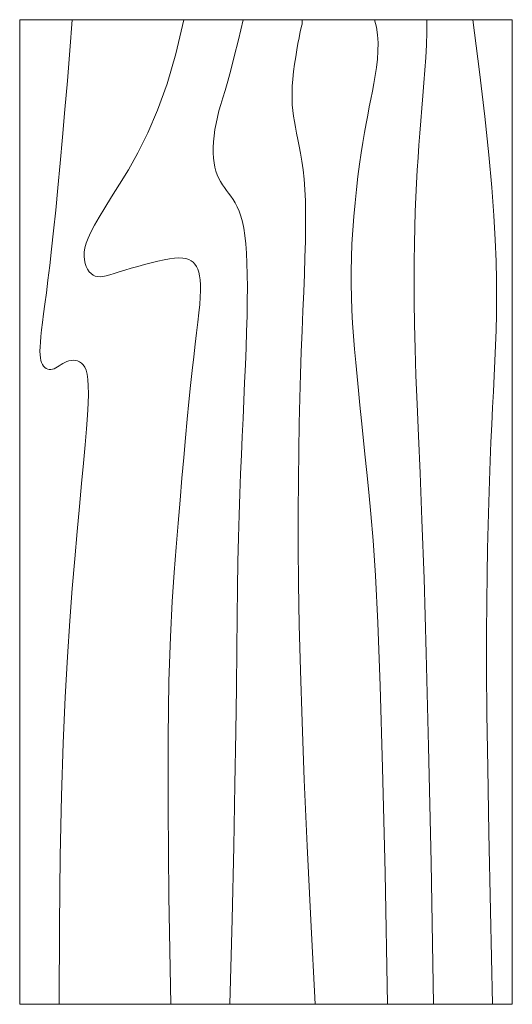
# Model space of a CAD drawing. Units: inches. Extents: x 3209 to 7144, y 1281 to 3076.
# Tile 5 of 5: x 7114 to 7144, y 3016 to 3076. Entities that reach past the tile are written whole.
import ezdxf

# ---------------------------------------------------------------- set-up
doc = ezdxf.new("R2010")
doc.units = ezdxf.units.IN
doc.layers.add('A-FURN', color=8, linetype='Continuous', lineweight=18)

# ---------------------------------------------------------------- blocks, each defined once
blk = doc.blocks.new('Table - Rectangular Woodgrain 60 x 30 in.')
for p, q in [((0, 0), (0, -30)), ((60, 0), (0, 0)), ((60, -30), (60, 0)), ((0, -30), (60, -30))]:
    blk.add_line(p, q)
for points in [[(0, -2.4), (4.8155, -2.418), (9.0302, -2.4688), (12.709, -2.5477), (15.9167, -2.65), (18.7181, -2.7711), (21.1781, -2.9063), (23.3616, -3.0508), (25.3333, -3.2), (27.1477, -3.3495), (28.8172, -3.4958), (30.3437, -3.636), (31.7291, -3.7667), (32.9756, -3.8849), (34.0849, -3.9875), (35.059, -4.0714), (35.9, -4.1334), (36.6114, -4.1711), (37.2041, -4.1854), (37.6906, -4.1779), (38.0833, -4.15), (38.3948, -4.1034), (38.6375, -4.0396), (38.8239, -3.9602), (38.9666, -3.8667), (39.0764, -3.7608), (39.1573, -3.6448), (39.2116, -3.521), (39.2416, -3.3917), (39.2498, -3.2593), (39.2385, -3.1261), (39.21, -2.9944), (39.1666, -2.8667), (39.111, -2.7447), (39.0468, -2.6281), (38.978, -2.5163), (38.9083, -2.4083), (38.8418, -2.3035), (38.7823, -2.201), (38.7337, -2.1001), (38.7, -2), (38.6844, -1.9003), (38.6875, -1.8021), (38.7094, -1.707), (38.75, -1.6167), (38.8094, -1.5326), (38.8875, -1.4563), (38.9844, -1.3893), (39.1, -1.3333), (39.2351, -1.2896), (39.3937, -1.2583), (39.5804, -1.2396), (39.8, -1.2333), (40.057, -1.2396), (40.3562, -1.2583), (40.7023, -1.2896), (41.1, -1.3333), (41.5547, -1.3895), (42.0755, -1.4573), (42.6721, -1.5361), (43.3542, -1.625), (44.1316, -1.7233), (45.014, -1.8302), (46.0114, -1.9449), (47.1333, -2.0667), (48.3862, -2.1947), (49.7625, -2.3281), (51.2513, -2.4663), (52.8416, -2.6083), (54.5226, -2.7535), (56.2833, -2.9011), (58.1127, -3.0501), (60, -3.2)], [(0, -9.2), (6.5759, -9.0858), (11.9385, -9.0365), (16.2527, -9.0418), (19.6833, -9.0917), (22.3952, -9.1759), (24.5531, -9.2844), (26.322, -9.4069), (27.8666, -9.5333), (29.3241, -9.6553), (30.7203, -9.7719), (32.0532, -9.8837), (33.3208, -9.9917), (34.5213, -10.0965), (35.6526, -10.199), (36.7128, -10.2999), (37.7, -10.4), (38.6129, -10.4996), (39.4531, -10.5969), (40.223, -10.6895), (40.925, -10.775), (41.5613, -10.8512), (42.1344, -10.9156), (42.6465, -10.966), (43.1, -11), (43.4976, -11.0158), (43.8437, -11.0136), (44.143, -10.9942), (44.4, -10.9583), (44.6195, -10.9069), (44.8062, -10.8406), (44.9648, -10.7603), (45.1, -10.6667), (45.2155, -10.5598), (45.3114, -10.4365), (45.3871, -10.2929), (45.4416, -10.125), (45.4743, -9.929), (45.4844, -9.7011), (45.4709, -9.4371), (45.4333, -9.1333), (45.3716, -8.7883), (45.2896, -8.4104), (45.1919, -8.0107), (45.0833, -7.6), (44.9685, -7.1893), (44.8521, -6.7896), (44.7388, -6.4117), (44.6333, -6.0667), (44.54, -5.7628), (44.4614, -5.4979), (44.4001, -5.2675), (44.3583, -5.0667), (44.3384, -4.8909), (44.3427, -4.7354), (44.3736, -4.5956), (44.4333, -4.4667), (44.5236, -4.3453), (44.6427, -4.2333), (44.7884, -4.1339), (44.9583, -4.05), (45.1501, -3.9849), (45.3614, -3.9417), (45.59, -3.9234), (45.8333, -3.9333), (46.0915, -3.9749), (46.3734, -4.0531), (46.6906, -4.1736), (47.0542, -4.3417), (47.4756, -4.5629), (47.9661, -4.8427), (48.5372, -5.1866), (49.2, -5.6), (49.9676, -6.0844), (50.8594, -6.625), (51.8965, -7.2031), (53.1, -7.8), (54.491, -8.3969), (56.0906, -8.975), (57.9199, -9.5156), (60, -10)], [(0, -12.8), (5.1847, -12.9322), (9.6213, -13.0323), (13.3963, -13.1059), (16.5958, -13.1583), (19.3063, -13.1952), (21.614, -13.2219), (23.6054, -13.2439), (25.3666, -13.2667), (26.9728, -13.2947), (28.4531, -13.3281), (29.8256, -13.3663), (31.1083, -13.4083), (32.3191, -13.4535), (33.476, -13.501), (34.597, -13.5501), (35.7, -13.6), (36.7984, -13.6497), (37.8875, -13.6979), (38.9578, -13.743), (40, -13.7833), (41.0047, -13.8174), (41.9625, -13.8438), (42.864, -13.8607), (43.7, -13.8667), (44.4631, -13.8604), (45.1552, -13.8417), (45.7801, -13.8104), (46.3416, -13.7667), (46.8439, -13.7104), (47.2906, -13.6417), (47.6858, -13.5604), (48.0333, -13.4667), (48.3375, -13.3608), (48.6042, -13.2448), (48.8396, -13.121), (49.05, -12.9917), (49.2417, -12.8593), (49.4208, -12.7261), (49.5937, -12.5944), (49.7667, -12.4667), (49.9452, -12.3451), (50.1323, -12.2313), (50.3303, -12.1268), (50.5416, -12.0333), (50.7686, -11.9524), (51.0135, -11.8854), (51.2788, -11.8341), (51.5666, -11.8), (51.8785, -11.7843), (52.2116, -11.7865), (52.562, -11.8059), (52.926, -11.8417), (53.2998, -11.8931), (53.6795, -11.9594), (54.0614, -12.0397), (54.4416, -12.1333), (54.8223, -12.2401), (55.2293, -12.3625), (55.6942, -12.5037), (56.2489, -12.6667), (56.9251, -12.8547), (57.7545, -13.0708), (58.7689, -13.3182), (60, -13.6)], [(0, -18), (5.124, -17.7273), (9.6609, -17.5057), (13.6705, -17.3303), (17.2125, -17.1958), (20.3467, -17.0973), (23.1328, -17.0297), (25.6307, -16.9878), (27.9, -16.9667), (29.9928, -16.9617), (31.9302, -16.9703), (33.7254, -16.9907), (35.3917, -17.0208), (36.9423, -17.0588), (38.3906, -17.1026), (39.7499, -17.1503), (41.0333, -17.2), (42.2519, -17.2496), (43.4073, -17.2969), (44.4986, -17.3395), (45.525, -17.375), (46.4858, -17.4012), (47.3802, -17.4156), (48.2074, -17.416), (48.9667, -17.4), (49.6583, -17.3662), (50.2872, -17.3167), (50.8595, -17.2547), (51.3812, -17.1833), (51.8584, -17.1057), (52.2971, -17.025), (52.7034, -16.9443), (53.0833, -16.8667), (53.443, -16.7951), (53.789, -16.7313), (54.128, -16.6768), (54.4666, -16.6334), (54.8115, -16.6024), (55.1693, -16.5854), (55.5465, -16.5841), (55.95, -16.6), (56.3828, -16.6337), (56.8346, -16.6823), (57.2915, -16.7418), (57.7396, -16.8084), (58.165, -16.878), (58.5539, -16.9469), (58.8924, -17.0111), (59.1666, -17.0667), (59.3679, -17.1107), (59.5078, -17.1438), (59.6032, -17.1675), (59.6708, -17.1833), (59.7275, -17.193), (59.7901, -17.1979), (59.8753, -17.1998), (60, -17.2)], [(0, -22.4), (8.0098, -22.2501), (14.4094, -22.1011), (19.4168, -21.9535), (23.25, -21.8083), (26.1269, -21.6663), (28.2656, -21.5281), (29.884, -21.3947), (31.2, -21.2667), (32.3967, -21.1448), (33.5172, -21.0292), (34.5697, -20.9198), (35.5625, -20.8167), (36.5037, -20.7198), (37.4015, -20.6292), (38.2642, -20.5448), (39.1, -20.4667), (39.9164, -20.3951), (40.7187, -20.3313), (41.5117, -20.2768), (42.3, -20.2333), (43.0883, -20.2024), (43.8812, -20.1854), (44.6836, -20.1841), (45.5, -20.2), (46.3328, -20.234), (47.1747, -20.2844), (48.0163, -20.3488), (48.8479, -20.425), (49.66, -20.5106), (50.4429, -20.6031), (51.1872, -20.7004), (51.8833, -20.8), (52.5246, -20.8999), (53.1166, -20.9995), (53.6681, -21.0983), (54.1875, -21.1958), (54.6834, -21.2919), (55.1646, -21.3859), (55.6394, -21.4777), (56.1167, -21.5667), (56.6028, -21.6515), (57.0961, -21.7266), (57.5929, -21.7852), (58.0896, -21.8208), (58.5823, -21.8268), (59.0674, -21.7964), (59.5412, -21.723), (60, -21.6)], [(0, -25.2), (8.6355, -25.0504), (15.7026, -24.9031), (21.4049, -24.7606), (25.9458, -24.625), (29.529, -24.4988), (32.3578, -24.3844), (34.6359, -24.284), (36.5667, -24.2), (38.3213, -24.1341), (39.9417, -24.0854), (41.437, -24.0523), (42.8167, -24.0333), (44.0901, -24.0268), (45.2667, -24.0313), (46.3557, -24.0451), (47.3667, -24.0667), (48.309, -24.0947), (49.1928, -24.1287), (50.0284, -24.168), (50.826, -24.2125), (51.5959, -24.2617), (52.3483, -24.3151), (53.0935, -24.3725), (53.8417, -24.4334), (54.6009, -24.497), (55.3699, -24.561), (56.1454, -24.6226), (56.9239, -24.6792), (57.7021, -24.7279), (58.4764, -24.7662), (59.2435, -24.7911), (60, -24.8)], [(0, -28.8), (5.6867, -28.6681), (10.45, -28.5698), (14.407, -28.5012), (17.675, -28.4584), (20.3711, -28.4374), (22.6125, -28.4344), (24.5164, -28.4455), (26.2, -28.4667), (27.762, -28.4947), (29.2276, -28.5281), (30.6033, -28.5663), (31.8958, -28.6084), (33.1118, -28.6535), (34.2578, -28.7011), (35.3405, -28.7501), (36.3666, -28.8), (37.3443, -28.8497), (38.288, -28.8974), (39.2137, -28.9412), (40.1375, -28.9792), (41.0753, -29.0093), (42.0432, -29.0297), (43.0572, -29.0384), (44.1333, -29.0333), (45.2936, -29.0114), (46.5843, -28.9641), (48.0579, -28.8816), (49.7666, -28.7542), (51.7629, -28.5721), (54.0989, -28.3255), (56.8272, -28.0048), (60, -27.6)]]:
    blk.add_lwpolyline(points)

msp = doc.modelspace()

# ---------------------------------------------------------------- block references
at = {"layer": 'A-FURN', "rotation": 90}
msp.add_blockref('Table - Rectangular Woodgrain 60 x 30 in.', (7114.198, 3015.876), dxfattribs=at)

doc.saveas('drawing.dxf')
